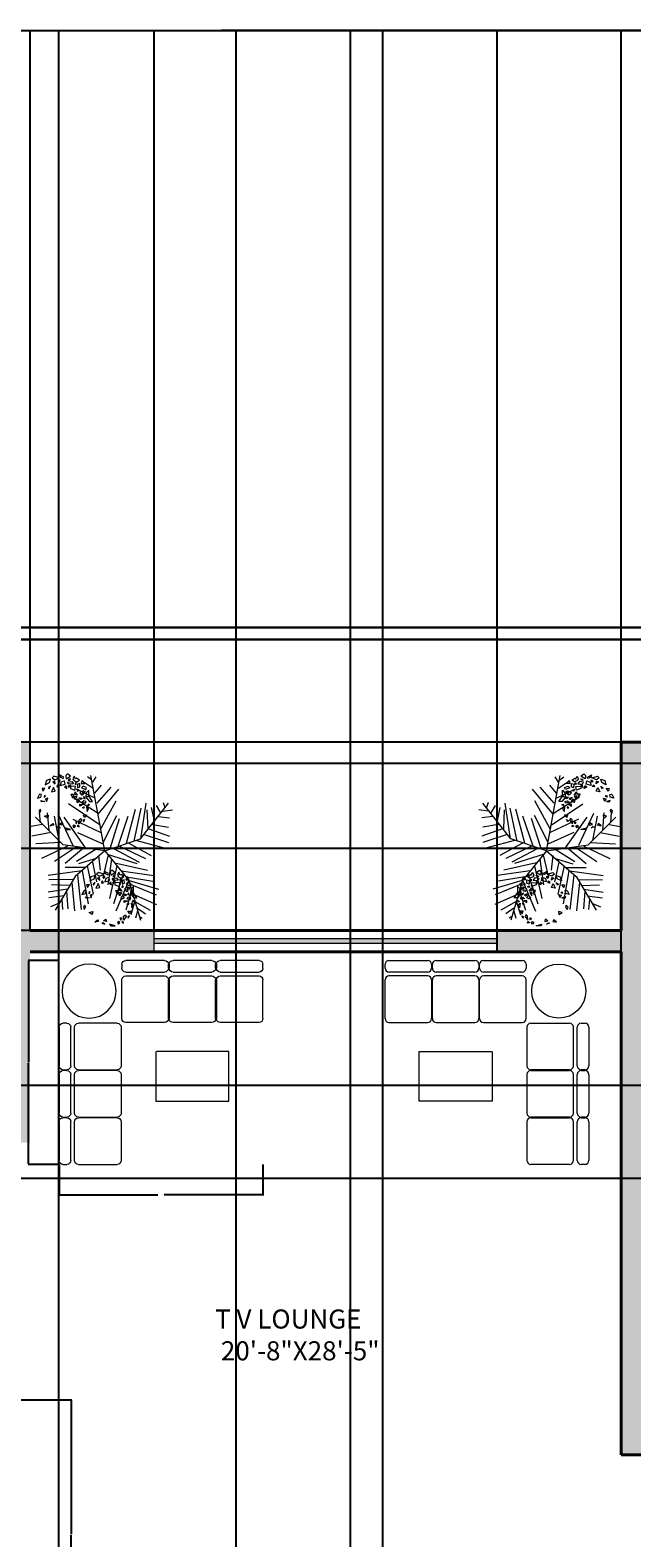
# Model space of a CAD drawing. Units: inches. Extents: x 2330 to 3943, y 1763 to 3461.
# Tile 25 of 40: x 2721 to 2973, y 2829 to 3461. Entities that reach past the tile are written whole.
import ezdxf

# ---------------------------------------------------------------- set-up
doc = ezdxf.new("R2010")
doc.units = ezdxf.units.IN
for name, color, linetype, lineweight in [('A-ANNO-DIMS', 2, 'Continuous', 18), ('A-AREA-IDEN', 7, 'Continuous', 18), ('A-FURN', 8, 'Continuous', 13), ('A-GLAZ', 4, 'Continuous', 18), ('A-WALL', 7, 'Continuous', 40), ('A-WALL-PATT', 252, 'Continuous', 13), ('C-PROP', 7, 'Continuous', 30), ('L-PLNT', 94, 'Continuous', 13)]:
    doc.layers.add(name, color=color, linetype=linetype, lineweight=lineweight)
doc.styles.get("Standard").update_dxf_attribs({"font": 'arial.ttf'})
doc.dimstyles.get("Standard").update_dxf_attribs({"dimtxt": 0.18, "dimasz": 0.18, "dimexe": 0.18, "dimexo": 0.0625, "dimgap": 0.09, "dimtad": 0, "dimtih": 1, "dimtoh": 1, "dimdec": 4, "dimzin": 0, "dimdsep": 46, "dimtxsty": 'Standard', "dimcen": 0.09, "dimadec": 0, "dimazin": 0, "dimtfac": 1, "dimtdec": 4, "dimtofl": 0, "dimtmove": 0, "dimatfit": 3, "dimfxl": 1, "dimtolj": 1, "dimtzin": 0, "dimarcsym": 0})

# ---------------------------------------------------------------- blocks, each defined once
blk = doc.blocks.new('A$C753D6792')
at = {"linetype": 'ByBlock'}
for p, q in [((0, 2530), (0, 2580)), ((50, 2630), (550, 2630)), ((600, 2580), (600, 2530)), ((610, 2530), (610, 2580)), ((660, 2630), (1160, 2630)), ((1210, 2580), (1210, 2530)), ((1220, 2530), (1220, 2580)), ((1270, 2630), (1770, 2630)), ((1820, 2580), (1820, 2530)), ((0, 1880), (0, 2380)), ((550, 2480), (50, 2480)), ((550, 2430), (50, 2430)), ((600, 2380), (600, 1880)), ((610, 1880), (610, 2380)), ((1160, 2480), (660, 2480)), ((1160, 2430), (660, 2430)), ((1210, 2380), (1210, 1880)), ((1220, 1880), (1220, 2380)), ((1770, 2480), (1270, 2480)), ((1770, 2430), (1270, 2430)), ((1820, 1880), (1820, 2380)), ((50, 1830), (427, 1830)), ((387, 1830), (550, 1830)), ((660, 1830), (1037, 1830)), ((997, 1830), (1160, 1830)), ((1270, 1830), (1647, 1830)), ((1607, 1830), (1770, 1830)), ((1830, 1770), (1830, 1393)), ((1880, 1820), (2380, 1820)), ((2430, 1270), (2430, 1770)), ((2480, 1270), (2480, 1770)), ((2530, 1820), (2580, 1820)), ((2630, 1770), (2630, 1270)), ((442, 815), (442, 1455)), ((442, 1455), (1372, 1455)), ((1382, 1455), (1382, 815)), ((1830, 1433), (1830, 1270)), ((2380, 1220), (1880, 1220)), ((1880, 1210), (2380, 1210)), ((2580, 1220), (2530, 1220)), ((2530, 1210), (2580, 1210)), ((1830, 1160), (1830, 783)), ((2430, 660), (2430, 1160)), ((2480, 660), (2480, 1160)), ((2630, 1160), (2630, 660)), ((1382, 815), (442, 815)), ((1830, 823), (1830, 660)), ((2380, 610), (1880, 610)), ((1880, 600), (2380, 600)), ((2580, 610), (2530, 610)), ((2530, 600), (2580, 600)), ((1830, 550), (1830, 173)), ((2430, 50), (2430, 550)), ((2480, 50), (2480, 550)), ((2630, 550), (2630, 50)), ((1830, 213), (1830, 50)), ((2380, 0), (1880, 0)), ((2580, 0), (2530, 0))]:
    blk.add_line(p, q, dxfattribs=at)
blk.add_circle((2242, 2235), 349, dxfattribs=at)
for centre, start, end in [((50, 2580), 90, 180), ((50, 2530), 180, 270), ((550, 2580), 0, 90), ((550, 2580), 0, 90), ((550, 2530), 270, 0), ((550, 2530), 270, 0), ((660, 2580), 90, 180), ((660, 2530), 180, 270), ((1160, 2580), 0, 90), ((1160, 2580), 0, 90), ((1160, 2530), 270, 0), ((1160, 2530), 270, 0), ((1270, 2580), 90, 180), ((1270, 2530), 180, 270), ((1770, 2580), 0, 90), ((1770, 2580), 0, 90), ((1770, 2530), 270, 0), ((1770, 2530), 270, 0), ((50, 2380), 90, 180), ((550, 2380), 0, 90), ((550, 2380), 0, 90), ((660, 2380), 90, 180), ((1160, 2380), 0, 90), ((1160, 2380), 0, 90), ((1270, 2380), 90, 180), ((1770, 2380), 0, 90), ((1770, 2380), 0, 90), ((50, 1880), 180, 270), ((550, 1880), 270, 0), ((660, 1880), 180, 270), ((1160, 1880), 270, 0), ((1270, 1880), 180, 270), ((1770, 1880), 270, 0), ((1880, 1770), 90, 180), ((2380, 1770), 0, 90), ((2530, 1770), 90, 180), ((2580, 1770), 0, 90), ((1880, 1270), 180, 270), ((1880, 1160), 90, 180), ((2380, 1270), 270, 0), ((2380, 1270), 270, 0), ((2380, 1160), 0, 90), ((2530, 1270), 180, 270), ((2530, 1270), 180, 270), ((2530, 1160), 90, 180), ((2580, 1270), 270, 0), ((2580, 1270), 270, 0), ((2580, 1160), 0, 90), ((1880, 660), 180, 270), ((1880, 550), 90, 180), ((2380, 660), 270, 0), ((2380, 660), 270, 0), ((2380, 550), 0, 90), ((2530, 660), 180, 270), ((2530, 660), 180, 270), ((2530, 550), 90, 180), ((2580, 660), 270, 0), ((2580, 660), 270, 0), ((2580, 550), 0, 90), ((1880, 50), 180, 270), ((2380, 50), 270, 0), ((2380, 50), 270, 0), ((2530, 50), 180, 270), ((2530, 50), 180, 270), ((2580, 50), 270, 0), ((2580, 50), 270, 0)]:
    blk.add_arc(centre, 50, start, end, dxfattribs=at)
blk = doc.blocks.new('*U12')
for p, q in [((0, 0), (-10.5, 57)), ((-7.288, 39.707), (-21.778, 46.673)), ((-8.737, 47.138), (-17.069, 52.711)), ((-10.186, 53.64), (-13.084, 55.962)), ((-9.099, 51.782), (-6.563, 55.962)), ((-7.65, 43.423), (-2.578, 49.46)), ((-5.839, 35.992), (4.667, 48.067)), ((-5.114, 27.632), (10.463, 46.673)), ((-3.665, 19.273), (-27.574, 35.527)), ((-5.114, 28.097), (-24.676, 40.636)), ((-2.941, 16.486), (8.652, 37.85)), ((27, 9), (48, 36)), ((27.127, 9.056), (31.112, 35.992)), ((44.153, 36.456), (45.239, 32.741)), ((-31.5, 4.5), (-52.5, 25.5)), ((-48.585, 21.131), (-49.309, 29.026)), ((-43.513, 28.561), (-42.427, 15.558)), ((-38.442, 26.239), (-34.819, 7.663)), ((-35.544, 28.097), (-24.314, 3.947)), ((-14.533, 2.09), (-30.834, 25.31)), ((-24.314, 23.917), (-2.941, 13.7)), ((-1.129, 6.734), (9.014, 26.704)), ((3.942, 1.625), (11.187, 24.381)), ((10.101, 3.483), (17.708, 26.239)), ((16.259, 5.805), (23.142, 31.348)), ((22.055, 7.198), (27.489, 32.277)), ((31.836, 30.883), (32.561, 16.486)), ((35.096, 32.741), (37.27, 22.524)), ((38.719, 34.134), (41.979, 28.561)), ((40.53, 25.775), (48.862, 24.846)), ((43.791, 29.954), (51.036, 30.883)), ((-47.498, 19.737), (-55.83, 18.344)), ((-40.615, 13.7), (-55.105, 10.913)), ((-20.691, 13.7), (-1.129, 4.876)), ((29.662, 12.307), (48.137, 6.269)), ((33.285, 16.486), (48.862, 10.913)), ((36.183, 19.737), (48.137, 17.88)), ((-33.37, 6.269), (-52.207, 5.34)), ((-28.299, 3.483), (-47.86, -5.805)), ((-21.416, 3.018), (-38.079, -8.128)), ((0, 0), (-31.5, 4.5)), ((-15.982, 2.09), (-30.11, -9.521)), ((0, 0), (-22.5, -19.5)), ((-6.563, 1.161), (-21.416, -8.128)), ((0, 0), (27, 9)), ((0, 0), (18, -22.5)), ((6.478, 1.625), (26.04, -8.592)), ((11.187, 3.483), (30.749, -5.805)), ((18.07, 5.805), (35.096, -3.483)), ((24.229, 7.663), (46.688, 1.625)), ((-6.563, -5.805), (-19.967, -9.985)), ((-13.446, -11.378), (-8.737, -32.741)), ((-9.461, -8.592), (-6.201, -23.453)), ((-4.752, -3.483), (-3.665, -14.629)), ((2.493, -3.019), (-1.491, -20.202)), ((1.769, -2.555), (24.229, -9.521)), ((5.029, -6.27), (2.131, -25.775)), ((9.014, -11.378), (3.58, -35.992)), ((7.565, -9.056), (32.198, -14.629)), ((-17.431, -15.094), (-42.789, -18.809)), ((-24.314, -21.596), (-42.427, -22.06)), ((-22.5, -19.5), (-37.5, -45)), ((-15.257, -12.772), (-30.11, -12.772)), ((-20.691, -18.345), (-17.793, -44.352)), ((-17.069, -15.094), (-12.721, -40.172)), ((14.085, -16.951), (6.478, -40.172)), ((18.07, -22.524), (8.289, -45.745)), ((12.274, -15.094), (36.907, -18.809)), ((16.259, -19.738), (36.183, -22.989)), ((18, -22.5), (27, -52.5)), ((18.433, -22.524), (40.53, -29.026)), ((-28.299, -29.026), (-42.789, -31.348)), ((-30.834, -34.135), (-42.427, -35.528)), ((-26.849, -26.24), (-40.253, -25.775)), ((-29.023, -30.884), (-27.936, -43.887)), ((-25.038, -23.918), (-22.865, -45.281)), ((20.244, -30.419), (15.897, -44.816)), ((19.157, -25.311), (38.719, -33.206)), ((21.331, -32.741), (39.081, -40.636)), ((-34.457, -39.708), (-40.978, -42.494)), ((-32.646, -36.921), (-31.921, -44.352)), ((22.78, -37.85), (19.519, -48.532)), ((22.78, -38.314), (34.372, -44.816)), ((24.591, -43.423), (30.749, -47.603)), ((24.591, -45.745), (23.142, -50.854)), ((26.764, -49.925), (28.213, -50.854))]:
    blk.add_line(p, q)
blk = doc.blocks.new('*U13')
for points in [[(-5.78, 9.75), (-7.54, 9.23), (-8.01, 7.5), (-6.26, 8.45)], [(-5.78, 6.81), (-6.66, 6.21), (-6.52, 5.69)], [(-4.57, 6.38), (-5.45, 4.47), (-3.89, 4.82)], [(-4.43, 11.05), (-5.18, 10.36), (-3.96, 9.49), (-2.07, 10.36)], [(-4.84, 8.63), (-3.83, 7.85), (-4.03, 8.97)], [(-2.88, 7.5), (-3.15, 6.64), (-2.27, 6.72)], [(-1.94, 9.49), (-2.48, 8.97), (-2.27, 8.54), (-1.8, 9.06)], [(-2, 11.66), (-1.6, 10.62), (-0.52, 10.1), (-0.18, 10.62), (-0.79, 10.96)], [(0.02, 9.06), (-1.33, 8.54), (-1.73, 7.16), (0.29, 7.76)], [(0.76, 7.16), (0.09, 6.46), (1.1, 5.95)], [(1.24, 12), (0.56, 11.31), (0.76, 10.01), (2.52, 11.05)], [(1.37, 8.54), (3.13, 8.8), (3.8, 7.85), (1.91, 7.76)], [(2.59, 9.93), (1.84, 9.75), (1.64, 9.23), (2.32, 9.41)], [(1.71, 6.29), (1.71, 7.07), (2.65, 7.5), (2.11, 6.9)], [(2.52, 6.81), (2.52, 5.86), (4.41, 5.17), (4.61, 6.72)], [(4.14, 11.14), (3.6, 10.01), (4, 9.23), (5.22, 8.71), (6.3, 9.41), (5.08, 10.19), (4.61, 10.01)], [(4.61, 8.28), (4.54, 7.76), (4.95, 7.59), (4.95, 8.28)], [(6.43, 7.94), (5.49, 7.68), (5.56, 6.21), (6.5, 6.64)], [(7.45, 9.32), (7.11, 7.94), (8.52, 7.94)], [(7.85, 6.81), (7.18, 6.21), (9, 5.51), (9.33, 6.38)], [(-11.32, 1.79), (-9.83, 2.31), (-9.63, 3.44), (-10.44, 3.52)], [(-8.21, 0.41), (-9.43, 0.32), (-9.83, 0.84)], [(-8.14, 6.03), (-9.36, 5.95), (-9.02, 4.73)], [(-8.21, 3.09), (-8.48, 2.31), (-7.87, 2.57)], [(-7, 1.79), (-7.94, 1.53), (-7.47, 0.49)], [(3.53, 1.88), (2.86, 3.52), (3.8, 3.52)], [(4.41, 4.56), (4.27, 3.7), (5.49, 3.26)], [(4.27, 2.74), (5.29, 2.66), (4.41, 1.27)], [(5.83, 1.53), (5.02, 0.41), (5.49, -0.02), (6.5, 0.41)], [(5.49, 5.51), (5.42, 4.82), (6.16, 5.08)], [(7.51, 1.71), (6.91, 1.27), (6.23, 2.14)], [(8.12, 4.99), (7.11, 4.65), (6.5, 4.13), (7.38, 3.09), (8.12, 3.52), (7.65, 3.87)], [(8.12, 0.75), (7.51, 0.15), (8.93, -0.28), (9.13, 0.49)], [(8.19, 2.57), (7.92, 2.05), (8.66, 1.53)], [(8.73, 4.73), (8.19, 4.56), (8.39, 3.87), (8.59, 4.04)], [(10.28, 5.17), (9.2, 4.04), (9, 2.31), (10.48, 0.49), (11.76, 0.41), (10.35, 2.48), (9.33, 2.4), (10.28, 2.83)], [(-10.03, -2.71), (-10.64, -3.31), (-10.44, -4.44), (-9.9, -3.49)], [(-8.28, -5.73), (-6.79, -5.3), (-7, -6.51)], [(7.78, -0.8), (6.43, -1.5), (6.43, -0.72)], [(8.32, -1.75), (7.98, -2.53), (7.58, -2.1)], [(9.33, -5.13), (8.46, -6.25), (7.98, -5.22)], [(9.33, -1.75), (9.54, -3.74), (10.14, -2.53)], [(10.08, -0.63), (9.74, -1.32), (10.48, -0.89)], [(-4.84, -8.85), (-4.43, -9.45), (-5.99, -9.8)], [(-2.54, -10.06), (-3.02, -10.23), (-1.8, -10.67)], [(-2.34, -9.2), (-1.26, -8.5), (-0.99, -9.54)], [(0.22, -10.58), (0.83, -11.27), (2.59, -11.36)], [(4.07, -9.45), (3.53, -9.97), (4.07, -10.58), (4.61, -9.89)], [(5.29, -7.98), (4.61, -8.16), (5.02, -8.94)], [(6.03, -9.45), (5.42, -9.97), (6.16, -10.15)], [(6.1, -8.94), (6.16, -7.21), (6.91, -6.69), (7.24, -7.38)], [(8.05, -8.07), (8.59, -7.12), (7.92, -7.55)]]:
    blk.add_lwpolyline(points, close=True)
blk = doc.blocks.new('*D41')
at = {"layer": 'A-ANNO-DIMS', "color": 0, "lineweight": -2, "transparency": 16777216}
for p, q in [((2732.81, 2985.45), (2732.81, 2972.51)), ((2818.34, 2985.45), (2818.34, 2972.51)), ((2732.99, 2972.69), (2774.21, 2972.69)), ((2818.16, 2972.69), (2776.95, 2972.69))]:
    blk.add_line(p, q, dxfattribs=at)
at = {"layer": 'A-ANNO-DIMS', "color": 0, "transparency": 16777216}
for points in [[(2732.99, 2972.72), (2732.99, 2972.66), (2732.81, 2972.69)], [(2818.16, 2972.72), (2818.16, 2972.66), (2818.34, 2972.69)]]:
    blk.add_solid(points, dxfattribs=at)
at = {"layer": 'Defpoints', "color": 0, "transparency": 16777216}
for p in [(2732.81, 2985.52), (2818.34, 2985.52), (2732.81, 2972.69)]:
    blk.add_point(p, dxfattribs=at)
at = {"layer": 'A-ANNO-DIMS', "color": 0, "transparency": 16777216, "insert": (2775.58, 2972.69), "char_height": 0.18, "attachment_point": 5}
blk.add_mtext('\\A1;LOUNGE SET 86 TYP.', dxfattribs=at)
blk = doc.blocks.new('*D42')
at = {"layer": 'A-ANNO-DIMS', "color": 0, "lineweight": -2, "transparency": 16777216}
for p, q in [((2732.75, 3071.05), (2719.8, 3071.05)), ((2719.98, 3070.87), (2719.98, 3028.47)), ((2719.98, 2985.7), (2719.98, 3028.1)), ((2732.75, 2985.52), (2719.8, 2985.52))]:
    blk.add_line(p, q, dxfattribs=at)
at = {"layer": 'A-ANNO-DIMS', "color": 0, "transparency": 16777216}
for points in [[(2719.95, 3070.87), (2720.01, 3070.87), (2719.98, 3071.05)], [(2719.95, 2985.7), (2720.01, 2985.7), (2719.98, 2985.52)]]:
    blk.add_solid(points, dxfattribs=at)
at = {"layer": 'Defpoints', "color": 0, "transparency": 16777216}
for p in [(2719.98, 3071.05), (2732.81, 3071.05), (2732.81, 2985.52)]:
    blk.add_point(p, dxfattribs=at)
at = {"layer": 'A-ANNO-DIMS', "color": 0, "transparency": 16777216, "insert": (2719.98, 3028.29), "char_height": 0.18, "attachment_point": 5}
blk.add_mtext('\\A1;86 TYP.', dxfattribs=at)
blk = doc.blocks.new('*D52')
at = {"layer": 'A-ANNO-DIMS', "color": 0, "lineweight": -2, "transparency": 16777216}
for p, q in [((2705.22, 2886.72), (2738.1, 2886.72)), ((2737.92, 2886.54), (2737.92, 2830.48)), ((2737.92, 2774.05), (2737.92, 2830.11)), ((2705.22, 2773.87), (2738.1, 2773.87))]:
    blk.add_line(p, q, dxfattribs=at)
at = {"layer": 'A-ANNO-DIMS', "color": 0, "transparency": 16777216}
for points in [[(2737.89, 2886.54), (2737.95, 2886.54), (2737.92, 2886.72)], [(2737.89, 2774.05), (2737.95, 2774.05), (2737.92, 2773.87)]]:
    blk.add_solid(points, dxfattribs=at)
at = {"layer": 'Defpoints', "color": 0, "transparency": 16777216}
for p in [(2705.15, 2886.72), (2737.92, 2886.72), (2705.15, 2773.87)]:
    blk.add_point(p, dxfattribs=at)
at = {"layer": 'A-ANNO-DIMS', "color": 0, "transparency": 16777216, "insert": (2737.92, 2830.3), "char_height": 0.18, "attachment_point": 5}
blk.add_mtext('\\A1;113', dxfattribs=at)
blk = doc.blocks.new('*D59')
at = {"layer": 'A-ANNO-DIMS', "color": 0, "lineweight": -2, "transparency": 16777216}
for p, q in [((2415.66, 3210.71), (2415.66, 3461.3)), ((2415.84, 3461.12), (3111.31, 3461.12)), ((3807.48, 3461.12), (3112.01, 3461.12)), ((3807.66, 3210.71), (3807.66, 3461.3))]:
    blk.add_line(p, q, dxfattribs=at)
at = {"layer": 'A-ANNO-DIMS', "color": 0, "transparency": 16777216}
for points in [[(2415.84, 3461.15), (2415.84, 3461.09), (2415.66, 3461.12)], [(3807.48, 3461.15), (3807.48, 3461.09), (3807.66, 3461.12)]]:
    blk.add_solid(points, dxfattribs=at)
at = {"layer": 'Defpoints', "color": 0, "transparency": 16777216}
for p in [(3807.66, 3461.12), (2415.66, 3210.65), (3807.66, 3210.65)]:
    blk.add_point(p, dxfattribs=at)
at = {"layer": 'A-ANNO-DIMS', "color": 0, "transparency": 16777216, "insert": (3111.66, 3461.12), "char_height": 0.18, "attachment_point": 5}
blk.add_mtext('\\A1;1392', dxfattribs=at)
blk = doc.blocks.new('*D61')
at = {"layer": 'A-ANNO-DIMS', "color": 0, "lineweight": -2, "transparency": 16777216}
for p, q in [((2475.66, 3162.71), (2475.66, 3461.3)), ((2475.84, 3461.12), (2965.37, 3461.12)), ((3455.48, 3461.12), (2965.95, 3461.12)), ((3455.66, 3162.71), (3455.66, 3461.3))]:
    blk.add_line(p, q, dxfattribs=at)
at = {"layer": 'A-ANNO-DIMS', "color": 0, "transparency": 16777216}
for points in [[(2475.84, 3461.15), (2475.84, 3461.09), (2475.66, 3461.12)], [(3455.48, 3461.15), (3455.48, 3461.09), (3455.66, 3461.12)]]:
    blk.add_solid(points, dxfattribs=at)
at = {"layer": 'Defpoints', "color": 0, "transparency": 16777216}
for p in [(3455.66, 3461.12), (2475.66, 3162.65), (3455.66, 3162.65)]:
    blk.add_point(p, dxfattribs=at)
at = {"layer": 'A-ANNO-DIMS', "color": 0, "transparency": 16777216, "insert": (2965.66, 3461.12), "char_height": 0.18, "attachment_point": 5}
blk.add_mtext('\\A1;980', dxfattribs=at)
blk = doc.blocks.new('*D72')
at = {"layer": 'A-ANNO-DIMS', "color": 0, "lineweight": -2, "transparency": 16777216}
for p, q in [((2732.66, 2712.71), (2732.66, 3461.3)), ((2732.84, 3461.12), (2800.38, 3461.12)), ((2868.48, 3461.12), (2800.94, 3461.12)), ((2868.66, 2712.71), (2868.66, 3461.3))]:
    blk.add_line(p, q, dxfattribs=at)
at = {"layer": 'A-ANNO-DIMS', "color": 0, "transparency": 16777216}
for points in [[(2732.84, 3461.15), (2732.84, 3461.09), (2732.66, 3461.12)], [(2868.48, 3461.15), (2868.48, 3461.09), (2868.66, 3461.12)]]:
    blk.add_solid(points, dxfattribs=at)
at = {"layer": 'Defpoints', "color": 0, "transparency": 16777216}
for p in [(2868.66, 3461.12), (2732.66, 2712.65), (2868.66, 2712.65)]:
    blk.add_point(p, dxfattribs=at)
at = {"layer": 'A-ANNO-DIMS', "color": 0, "transparency": 16777216, "insert": (2800.66, 3461.12), "char_height": 0.18, "attachment_point": 5}
blk.add_mtext('\\A1;136', dxfattribs=at)
blk = doc.blocks.new('*D74')
at = {"layer": 'A-ANNO-DIMS', "color": 0, "lineweight": -2, "transparency": 16777216}
for p, q in [((2807.16, 2457.71), (2807.16, 3461.3)), ((2807.34, 3461.12), (2830.94, 3461.12)), ((2854.98, 3461.12), (2831.38, 3461.12)), ((2855.16, 2457.71), (2855.16, 3461.3))]:
    blk.add_line(p, q, dxfattribs=at)
at = {"layer": 'A-ANNO-DIMS', "color": 0, "transparency": 16777216}
for points in [[(2807.34, 3461.15), (2807.34, 3461.09), (2807.16, 3461.12)], [(2854.98, 3461.15), (2854.98, 3461.09), (2855.16, 3461.12)]]:
    blk.add_solid(points, dxfattribs=at)
at = {"layer": 'Defpoints', "color": 0, "transparency": 16777216}
for p in [(2855.16, 3461.12), (2807.16, 2457.65), (2855.16, 2457.65)]:
    blk.add_point(p, dxfattribs=at)
at = {"layer": 'A-ANNO-DIMS', "color": 0, "transparency": 16777216, "insert": (2831.16, 3461.12), "char_height": 0.18, "attachment_point": 5}
blk.add_mtext('\\A1;48', dxfattribs=at)
blk = doc.blocks.new('*D75')
at = {"layer": 'A-ANNO-DIMS', "color": 0, "lineweight": -2, "transparency": 16777216}
for p, q in [((2720.66, 3083.71), (2720.66, 3461.3)), ((2720.84, 3461.12), (2844.37, 3461.12)), ((2968.48, 3461.12), (2844.95, 3461.12)), ((2968.66, 3083.71), (2968.66, 3461.3))]:
    blk.add_line(p, q, dxfattribs=at)
at = {"layer": 'A-ANNO-DIMS', "color": 0, "transparency": 16777216}
for points in [[(2720.84, 3461.15), (2720.84, 3461.09), (2720.66, 3461.12)], [(2968.48, 3461.15), (2968.48, 3461.09), (2968.66, 3461.12)]]:
    blk.add_solid(points, dxfattribs=at)
at = {"layer": 'Defpoints', "color": 0, "transparency": 16777216}
for p in [(2968.66, 3461.12), (2720.66, 3083.65), (2968.66, 3083.65)]:
    blk.add_point(p, dxfattribs=at)
at = {"layer": 'A-ANNO-DIMS', "color": 0, "transparency": 16777216, "insert": (2844.66, 3461.12), "char_height": 0.18, "attachment_point": 5}
blk.add_mtext('\\A1;248', dxfattribs=at)
blk = doc.blocks.new('*D76')
at = {"layer": 'A-ANNO-DIMS', "color": 0, "lineweight": -2, "transparency": 16777216}
for p, q in [((2968.6, 3162.65), (2330.5, 3162.65)), ((2330.68, 3162.47), (2330.68, 3123.33)), ((2330.68, 3083.83), (2330.68, 3122.97)), ((2968.6, 3083.65), (2330.5, 3083.65))]:
    blk.add_line(p, q, dxfattribs=at)
at = {"layer": 'A-ANNO-DIMS', "color": 0, "transparency": 16777216}
for points in [[(2330.65, 3162.47), (2330.71, 3162.47), (2330.68, 3162.65)], [(2330.65, 3083.83), (2330.71, 3083.83), (2330.68, 3083.65)]]:
    blk.add_solid(points, dxfattribs=at)
at = {"layer": 'Defpoints', "color": 0, "transparency": 16777216}
for p in [(2330.68, 3162.65), (2968.66, 3162.65), (2968.66, 3083.65)]:
    blk.add_point(p, dxfattribs=at)
at = {"layer": 'A-ANNO-DIMS', "color": 0, "transparency": 16777216, "insert": (2330.68, 3123.15), "char_height": 0.18, "attachment_point": 5}
blk.add_mtext('\\A1;79', dxfattribs=at)
blk = doc.blocks.new('*D85')
at = {"layer": 'A-ANNO-DIMS', "color": 0, "lineweight": -2, "transparency": 16777216}
for p, q in [((3091.6, 3153.65), (2330.5, 3153.65)), ((2330.68, 3153.47), (2330.68, 3136.04)), ((2330.68, 3118.24), (2330.68, 3135.67)), ((3091.6, 3118.06), (2330.5, 3118.06))]:
    blk.add_line(p, q, dxfattribs=at)
at = {"layer": 'A-ANNO-DIMS', "color": 0, "transparency": 16777216}
for points in [[(2330.65, 3153.47), (2330.71, 3153.47), (2330.68, 3153.65)], [(2330.65, 3118.24), (2330.71, 3118.24), (2330.68, 3118.06)]]:
    blk.add_solid(points, dxfattribs=at)
at = {"layer": 'Defpoints', "color": 0, "transparency": 16777216}
for p in [(2330.68, 3153.65), (3091.66, 3153.65), (3091.66, 3118.06)]:
    blk.add_point(p, dxfattribs=at)
at = {"layer": 'A-ANNO-DIMS', "color": 0, "transparency": 16777216, "insert": (2330.68, 3135.86), "char_height": 0.18, "attachment_point": 5}
blk.add_mtext('\\A1;35.59', dxfattribs=at)
blk = doc.blocks.new('*D91')
at = {"layer": 'A-ANNO-DIMS', "color": 0, "lineweight": -2, "transparency": 16777216}
for p, q in [((2772.66, 3083.71), (2772.66, 3461.3)), ((2772.84, 3461.12), (2844.38, 3461.12)), ((2916.48, 3461.12), (2844.94, 3461.12)), ((2916.66, 3083.71), (2916.66, 3461.3))]:
    blk.add_line(p, q, dxfattribs=at)
at = {"layer": 'A-ANNO-DIMS', "color": 0, "transparency": 16777216}
for points in [[(2772.84, 3461.15), (2772.84, 3461.09), (2772.66, 3461.12)], [(2916.48, 3461.15), (2916.48, 3461.09), (2916.66, 3461.12)]]:
    blk.add_solid(points, dxfattribs=at)
at = {"layer": 'Defpoints', "color": 0, "transparency": 16777216}
for p in [(2916.66, 3461.12), (2772.66, 3083.65), (2916.66, 3083.65)]:
    blk.add_point(p, dxfattribs=at)
at = {"layer": 'A-ANNO-DIMS', "color": 0, "transparency": 16777216, "insert": (2844.66, 3461.12), "char_height": 0.18, "attachment_point": 5}
blk.add_mtext('\\A1;144', dxfattribs=at)
blk = doc.blocks.new('*D92')
at = {"layer": 'A-ANNO-DIMS', "color": 0, "lineweight": -2, "transparency": 16777216}
for p, q in [((2916.66, 3074.71), (2916.66, 3461.3)), ((2916.84, 3461.12), (2942.44, 3461.12)), ((2968.48, 3461.12), (2942.88, 3461.12)), ((2968.66, 3074.71), (2968.66, 3461.3))]:
    blk.add_line(p, q, dxfattribs=at)
at = {"layer": 'A-ANNO-DIMS', "color": 0, "transparency": 16777216}
for points in [[(2916.84, 3461.15), (2916.84, 3461.09), (2916.66, 3461.12)], [(2968.48, 3461.15), (2968.48, 3461.09), (2968.66, 3461.12)]]:
    blk.add_solid(points, dxfattribs=at)
at = {"layer": 'Defpoints', "color": 0, "transparency": 16777216}
for p in [(2968.66, 3461.12), (2916.66, 3074.65), (2968.66, 3074.65)]:
    blk.add_point(p, dxfattribs=at)
at = {"layer": 'A-ANNO-DIMS', "color": 0, "transparency": 16777216, "insert": (2942.66, 3461.12), "char_height": 0.18, "attachment_point": 5}
blk.add_mtext('\\A1;52', dxfattribs=at)
blk = doc.blocks.new('*D93')
at = {"layer": 'A-ANNO-DIMS', "color": 0, "lineweight": -2, "transparency": 16777216}
for p, q in [((3446.6, 3018.65), (2330.5, 3018.65)), ((2330.68, 3018.47), (2330.68, 2999.33)), ((2330.68, 2979.83), (2330.68, 2998.97)), ((3446.6, 2979.65), (2330.5, 2979.65))]:
    blk.add_line(p, q, dxfattribs=at)
at = {"layer": 'A-ANNO-DIMS', "color": 0, "transparency": 16777216}
for points in [[(2330.65, 3018.47), (2330.71, 3018.47), (2330.68, 3018.65)], [(2330.65, 2979.83), (2330.71, 2979.83), (2330.68, 2979.65)]]:
    blk.add_solid(points, dxfattribs=at)
at = {"layer": 'Defpoints', "color": 0, "transparency": 16777216}
for p in [(2330.68, 3018.65), (3446.66, 3018.65), (3446.66, 2979.65)]:
    blk.add_point(p, dxfattribs=at)
at = {"layer": 'A-ANNO-DIMS', "color": 0, "transparency": 16777216, "insert": (2330.68, 2999.15), "char_height": 0.18, "attachment_point": 5}
blk.add_mtext('\\A1;39', dxfattribs=at)

msp = doc.modelspace()

# ---------------------------------------------------------------- hatches: boundary and pattern name
at = {"layer": 'A-GLAZ'}
h = msp.add_hatch(color=256, dxfattribs=at)
h.dxf.hatch_style = 1
h.paths.add_polyline_path([(2916.6605, 3080.1524), (2772.6605, 3080.1524), (2772.6605, 3078.1524), (2916.6605, 3078.1524)])
at = {"layer": 'A-WALL-PATT'}
h = msp.add_hatch(color=256, dxfattribs=at)
h.dxf.hatch_style = 1
h.paths.add_polyline_path([(2772.6605, 3083.6524), (2720.6605, 3083.6524), (2720.6605, 3162.6524), (2678.6605, 3162.6524), (2678.6605, 3153.6524), (2711.6605, 3153.6524), (2711.6605, 2994.6524), (2720.6605, 2994.6524), (2720.6605, 3074.6524), (2772.6605, 3074.6524)])
h = msp.add_hatch(color=256, dxfattribs=at)
h.dxf.hatch_style = 1
h.paths.add_polyline_path([(3022.6605, 3162.6524), (2968.6605, 3162.6524), (2968.6605, 3083.6524), (2916.6605, 3083.6524), (2916.6605, 3074.6524), (2968.6605, 3074.6524), (2968.6605, 2863.6524), (2977.6605, 2863.6524), (2977.6605, 2867.6524), (3096.6605, 2867.6524), (3096.6605, 2913.1524), (3114.6605, 2913.1524), (3114.6605, 2918.1524), (3096.6605, 2918.1524), (3096.6605, 2958.6524), (3091.6605, 2958.6524), (3091.6605, 2872.6524), (2977.6605, 2872.6524), (2977.6605, 2998.6524), (3057.6605, 2998.6524), (3057.6605, 3003.6524), (2977.6605, 3003.6524), (2977.6605, 3153.6524), (3022.6605, 3153.6524)])

# ---------------------------------------------------------------- linework, layer by layer
at = {"layer": 'A-GLAZ'}
for p, q in [((2772.6605, 3074.6524), (2772.6605, 3083.6524)), ((2916.6605, 3080.1524), (2772.6605, 3080.1524)), ((2916.6605, 3074.6524), (2916.6605, 3083.6524)), ((2916.6605, 3078.1524), (2772.6605, 3078.1524))]:
    msp.add_line(p, q, dxfattribs=at)
at = {"layer": 'A-WALL'}
for p, q in [((2968.6605, 3162.6524), (2968.6605, 3083.6524)), ((2968.6605, 3162.6524), (3455.6605, 3162.6524)), ((2720.6605, 3083.6524), (2968.6605, 3083.6524)), ((2720.6605, 3074.6524), (2968.6605, 3074.6524)), ((2968.6605, 3074.6524), (2968.6605, 2863.6524)), ((2968.6605, 2863.6524), (2977.6605, 2863.6524))]:
    msp.add_line(p, q, dxfattribs=at)
at = {"layer": 'C-PROP'}
for p, q in [((2415.6605, 3210.6524), (3807.6605, 3210.6524)), ((2420.6605, 3205.6524), (3802.6605, 3205.6524))]:
    msp.add_line(p, q, dxfattribs=at)

# ---------------------------------------------------------------- block references
at = {"layer": 'A-FURN', "yscale": 0.0325230000849776, "zscale": 0.0325230000849776}
for p, xscale in [((2818.3449, 2985.5175), -0.0325230000849776), ((2869.5957, 2985.5175), 0.0325230000849776)]:
    msp.add_blockref('A$C753D6792', p, dxfattribs=dict(at, xscale=xscale))
at = {"layer": 'L-PLNT', "yscale": 0.5550642544959848, "zscale": 0.5550642544959848}
for p, xscale in [((2752.017, 3117.0641), 0.5550642544959848), ((2937.3041, 3117.0641), -0.5550642544959848)]:
    msp.add_blockref('*U12', p, dxfattribs=dict(at, xscale=xscale))
at = {"layer": 'L-PLNT'}
for p in [(2735.0268, 3137.2841), (2753.7338, 3096.8862)]:
    msp.add_blockref('*U13', p, dxfattribs=at)
at = {"layer": 'L-PLNT', "xscale": -1}
for p in [(2954.2943, 3137.2841), (2935.5872, 3096.8862)]:
    msp.add_blockref('*U13', p, dxfattribs=at)

# ---------------------------------------------------------------- texts
at = {"layer": 'A-AREA-IDEN', "insert": (2795.814, 2924.6364), "char_height": 8, "attachment_point": 1}
msp.add_mtext_dynamic_manual_height_columns(' T V LOUNGE\\P  20\'-8"X28\'-5"', width=103.554571, gutter_width=12.5, heights=[0], dxfattribs=at)

# ---------------------------------------------------------------- dimensions: what is measured, and where the dimension line sits
at = {"layer": 'A-ANNO-DIMS'}
for base, p1, p2, picture, middle in [((3807.6605, 3461.1231), (2415.6605, 3210.6524), (3807.6605, 3210.6524), '*D59', (3111.6605, 3461.1231)), ((3455.6605, 3461.1231), (2475.6605, 3162.6524), (3455.6605, 3162.6524), '*D61', (2965.6605, 3461.1231)), ((2968.6605, 3461.1231), (2720.6605, 3083.6524), (2968.6605, 3083.6524), '*D75', (2844.6605, 3461.1231)), ((2868.6605, 3461.1231), (2732.6605, 2712.6524), (2868.6605, 2712.6524), '*D72', (2800.6605, 3461.1231)), ((2916.6605, 3461.1231), (2772.6605, 3083.6524), (2916.6605, 3083.6524), '*D91', (2844.6605, 3461.1231)), ((2855.1605, 3461.1231), (2807.1605, 2457.6524), (2855.1605, 2457.6524), '*D74', (2831.1605, 3461.1231)), ((2968.6605, 3461.1231), (2916.6605, 3074.6524), (2968.6605, 3074.6524), '*D92', (2942.6605, 3461.1231))]:
    dim = msp.add_linear_dim(base=base, p1=p1, p2=p2, dimstyle='Standard', override={"dimdec": 0, "dimlfac": 1, "dimrnd": 0, "dimzin": 0, "dimdsep": 46, "dimlunit": 2}, dxfattribs=at)
    dim.commit()
    dim.dimension.update_dxf_attribs({"geometry": picture, "text_midpoint": middle})
for base, p1, p2, override, picture, middle in [((2330.6824, 3162.6524), (2968.6605, 3083.6524), (2968.6605, 3162.6524), {"dimdec": 0, "dimlfac": 1, "dimrnd": 0, "dimzin": 0, "dimdsep": 46, "dimlunit": 2}, '*D76', (2330.6824, 3123.1524)), ((2330.6824, 3153.6524), (3091.6605, 3118.0598), (3091.6605, 3153.6524), {"dimdec": 2, "dimlfac": 1, "dimrnd": 0, "dimzin": 0, "dimdsep": 46, "dimlunit": 2}, '*D85', (2330.6824, 3135.8561)), ((2330.6824, 3018.6524), (3446.6605, 2979.6524), (3446.6605, 3018.6524), {"dimdec": 0, "dimlfac": 1, "dimrnd": 0, "dimzin": 0, "dimdsep": 46, "dimlunit": 2}, '*D93', (2330.6824, 2999.1524)), ((2737.9166, 2886.7243), (2705.1545, 2773.8664), (2705.1545, 2886.7243), {"dimdec": 0, "dimlfac": 1, "dimrnd": 0, "dimzin": 0, "dimdsep": 46, "dimlunit": 2}, '*D52', (2737.9166, 2830.2954))]:
    dim = msp.add_linear_dim(base=base, p1=p1, p2=p2, angle=90, dimstyle='Standard', override=override, dxfattribs=at)
    dim.commit()
    dim.dimension.update_dxf_attribs({"geometry": picture, "text_midpoint": middle})
for base, p1, p2, angle, text, picture, middle in [((2719.9791, 3071.053), (2732.8094, 2985.5175), (2732.8094, 3071.053), 90, '<> TYP.', '*D42', (2719.9791, 3028.2852)), ((2732.8094, 2972.6872), (2818.3449, 2985.5175), (2732.8094, 2985.5175), 180, 'LOUNGE SET <> TYP.', '*D41', (2775.5772, 2972.6872))]:
    dim = msp.add_linear_dim(base=base, p1=p1, p2=p2, angle=angle, text=text, dimstyle='Standard', override={"dimdec": 0, "dimlfac": 1, "dimrnd": 0, "dimzin": 0, "dimdsep": 46, "dimlunit": 2}, dxfattribs=at)
    dim.commit()
    dim.dimension.update_dxf_attribs({"geometry": picture, "text_midpoint": middle})

doc.saveas('drawing.dxf')
